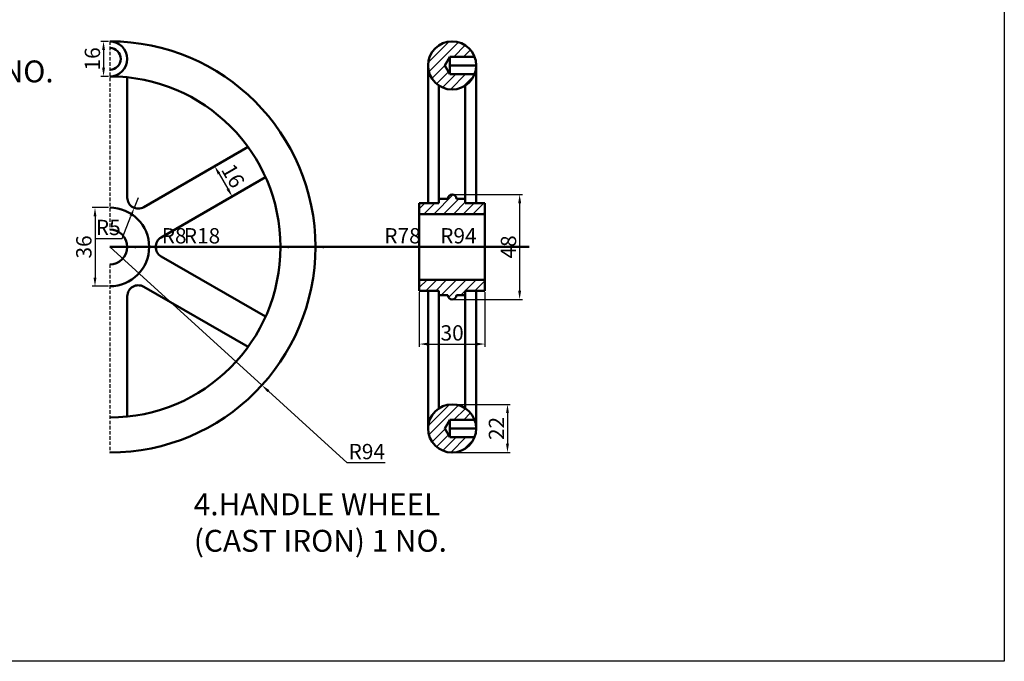
# Model space of a CAD drawing. Units: millimetres. Extents: x -66 to 1195, y -396 to 398.
# Tile 6 of 8: x 745 to 1195, y -396 to -102. Entities that reach past the tile are written whole.
import ezdxf

# ---------------------------------------------------------------- set-up
doc = ezdxf.new("R2010")
doc.units = ezdxf.units.MM
doc.header["$LTSCALE"] = 0.5
doc.linetypes.add('HIDDEN', pattern=[9.525, 6.35, -3.175])
for name, color, linetype, lineweight in [('M-DIMS', 2, 'Continuous', 25), ('M-HATC', 8, 'Continuous', 18), ('M-HIDN', 3, 'HIDDEN', 25), ('M-OUTL', 7, 'Continuous', 50), ('M-TEXT', 7, 'Continuous', 25), ('M-TTLB', 7, 'Continuous', 25)]:
    doc.layers.add(name, color=color, linetype=linetype, lineweight=lineweight)
doc.styles.get("Standard").update_dxf_attribs({"font": 'arial.ttf'})
doc.dimstyles.new('ISO-25', dxfattribs={"dimtxt": 7, "dimasz": 4, "dimexe": 1.25, "dimexo": 0.625, "dimtad": 1, "dimtoh": 1, "dimtxsty": 'Standard', "dimcen": 2.5, "dimadec": 0, "dimazin": 0, "dimtfac": 1, "dimtmove": 0, "dimatfit": 3, "dimfxl": 1, "dimarcsym": 0})

# ---------------------------------------------------------------- blocks, each defined once
blk = doc.blocks.new('*D89')
at = {"layer": 'Defpoints', "color": 0, "ltscale": 0.5, "transparency": 16777216}
for p in [(942.6, -182.22), (942.6, -230.22), (973.48, -230.22)]:
    blk.add_point(p, dxfattribs=at)
at = {"layer": 'M-DIMS', "color": 0, "lineweight": -2, "ltscale": 0.5, "transparency": 16777216}
for p, q in [((943.23, -182.22), (974.73, -182.22)), ((973.48, -186.22), (973.48, -226.22)), ((943.23, -230.22), (974.73, -230.22))]:
    blk.add_line(p, q, dxfattribs=at)
at = {"layer": 'M-DIMS', "color": 0, "ltscale": 0.5, "transparency": 16777216}
for points in [[(972.81, -186.22), (974.15, -186.22), (973.48, -182.22)], [(972.81, -226.22), (974.15, -226.22), (973.48, -230.22)]]:
    blk.add_solid(points, dxfattribs=at)
at = {"layer": 'M-DIMS', "color": 0, "ltscale": 0.5, "transparency": 16777216, "insert": (969.28, -206.22), "char_height": 7, "attachment_point": 5, "rotation": 90}
blk.add_mtext('48', dxfattribs=at)
blk = doc.blocks.new('*D90')
at = {"layer": 'Defpoints', "color": 0, "ltscale": 0.5, "transparency": 16777216}
for p in [(927.6, -226.22), (957.6, -226.22), (957.6, -250.62)]:
    blk.add_point(p, dxfattribs=at)
at = {"layer": 'M-DIMS', "color": 0, "lineweight": -2, "ltscale": 0.5, "transparency": 16777216}
for p, q in [((927.6, -226.84), (927.6, -251.87)), ((957.6, -226.84), (957.6, -251.87)), ((931.6, -250.62), (953.6, -250.62))]:
    blk.add_line(p, q, dxfattribs=at)
at = {"layer": 'M-DIMS', "color": 0, "ltscale": 0.5, "transparency": 16777216}
for points in [[(931.6, -249.95), (931.6, -251.28), (927.6, -250.62)], [(953.6, -249.95), (953.6, -251.28), (957.6, -250.62)]]:
    blk.add_solid(points, dxfattribs=at)
at = {"layer": 'M-DIMS', "color": 0, "ltscale": 0.5, "transparency": 16777216, "insert": (942.6, -246.42), "char_height": 7, "attachment_point": 5}
blk.add_mtext('30', dxfattribs=at)
blk = doc.blocks.new('*D91')
at = {"layer": 'Defpoints', "color": 0, "ltscale": 0.5, "transparency": 16777216}
for p in [(942.6, -278.22), (942.6, -300.22), (967.92, -300.22)]:
    blk.add_point(p, dxfattribs=at)
at = {"layer": 'M-DIMS', "color": 0, "lineweight": -2, "ltscale": 0.5, "transparency": 16777216}
for p, q in [((943.23, -278.22), (969.17, -278.22)), ((967.92, -282.22), (967.92, -296.22)), ((943.23, -300.22), (969.17, -300.22))]:
    blk.add_line(p, q, dxfattribs=at)
at = {"layer": 'M-DIMS', "color": 0, "ltscale": 0.5, "transparency": 16777216}
for points in [[(967.25, -282.22), (968.58, -282.22), (967.92, -278.22)], [(967.25, -296.22), (968.58, -296.22), (967.92, -300.22)]]:
    blk.add_solid(points, dxfattribs=at)
at = {"layer": 'M-DIMS', "color": 0, "ltscale": 0.5, "transparency": 16777216, "insert": (963.78, -289.22), "char_height": 7, "attachment_point": 5, "rotation": 90}
blk.add_mtext('22', dxfattribs=at)
blk = doc.blocks.new('*D92')
at = {"layer": 'Defpoints', "color": 0, "ltscale": 0.5, "transparency": 16777216}
for p in [(786.1, -206.22), (855.65, -269.46)]:
    blk.add_point(p, dxfattribs=at)
at = {"layer": 'M-DIMS', "color": 0, "lineweight": -2, "ltscale": 0.5, "transparency": 16777216}
for p, q in [((786.1, -206.22), (855.65, -269.46)), ((894.62, -304.9), (858.61, -272.15)), ((911.94, -304.9), (894.62, -304.9))]:
    blk.add_line(p, q, dxfattribs=at)
at = {"layer": 'M-DIMS', "color": 0, "ltscale": 0.5, "transparency": 16777216}
blk.add_solid([(859.05, -271.66), (858.16, -272.64), (855.65, -269.46)], dxfattribs=at)
at = {"layer": 'M-DIMS', "color": 0, "ltscale": 0.5, "transparency": 16777216, "insert": (903.59, -300.7), "char_height": 7, "attachment_point": 5}
blk.add_mtext('R94', dxfattribs=at)
blk = doc.blocks.new('*D93')
at = {"layer": 'Defpoints', "color": 0, "ltscale": 0.5, "transparency": 16777216}
for p in [(825.45, -174.26), (842.05, -183.15), (833.45, -188.12)]:
    blk.add_point(p, dxfattribs=at)
at = {"layer": 'M-DIMS', "color": 0, "lineweight": -2, "ltscale": 0.5, "transparency": 16777216}
for p, q in [((825.99, -173.95), (835.13, -168.67)), ((836.05, -172.76), (840.05, -179.69)), ((833.99, -187.81), (843.13, -182.53))]:
    blk.add_line(p, q, dxfattribs=at)
at = {"layer": 'M-DIMS', "color": 0, "ltscale": 0.5, "transparency": 16777216}
for points in [[(836.63, -172.43), (835.47, -173.1), (834.05, -169.3)], [(840.63, -179.36), (839.47, -180.02), (842.05, -183.15)]]:
    blk.add_solid(points, dxfattribs=at)
at = {"layer": 'M-DIMS', "color": 0, "ltscale": 0.5, "transparency": 16777216, "insert": (841.69, -174.13), "char_height": 7, "attachment_point": 5, "rotation": 300}
blk.add_mtext('16', dxfattribs=at)
blk = doc.blocks.new('*D94')
at = {"layer": 'Defpoints', "color": 0, "ltscale": 0.5, "transparency": 16777216}
for p in [(786.1, -188.22), (779.34, -224.22), (786.1, -224.22)]:
    blk.add_point(p, dxfattribs=at)
at = {"layer": 'M-DIMS', "color": 0, "lineweight": -2, "ltscale": 0.5, "transparency": 16777216}
for p, q in [((785.48, -188.22), (778.09, -188.22)), ((779.34, -192.22), (779.34, -220.22)), ((785.48, -224.22), (778.09, -224.22))]:
    blk.add_line(p, q, dxfattribs=at)
at = {"layer": 'M-DIMS', "color": 0, "ltscale": 0.5, "transparency": 16777216}
for points in [[(778.67, -192.22), (780, -192.22), (779.34, -188.22)], [(778.67, -220.22), (780, -220.22), (779.34, -224.22)]]:
    blk.add_solid(points, dxfattribs=at)
at = {"layer": 'M-DIMS', "color": 0, "ltscale": 0.5, "transparency": 16777216, "insert": (775.14, -206.22), "char_height": 7, "attachment_point": 5, "rotation": 90}
blk.add_mtext('36', dxfattribs=at)
blk = doc.blocks.new('*D95')
at = {"layer": 'Defpoints', "color": 0, "ltscale": 0.5, "transparency": 16777216}
for p in [(786.1, -112.22), (783.24, -128.22), (786.1, -128.22)]:
    blk.add_point(p, dxfattribs=at)
at = {"layer": 'M-DIMS', "color": 0, "lineweight": -2, "ltscale": 0.5, "transparency": 16777216}
for p, q in [((785.48, -112.22), (781.99, -112.22)), ((783.24, -116.22), (783.24, -124.22)), ((785.48, -128.22), (781.99, -128.22))]:
    blk.add_line(p, q, dxfattribs=at)
at = {"layer": 'M-DIMS', "color": 0, "ltscale": 0.5, "transparency": 16777216}
for points in [[(782.58, -116.22), (783.91, -116.22), (783.24, -112.22)], [(782.58, -124.22), (783.91, -124.22), (783.24, -128.22)]]:
    blk.add_solid(points, dxfattribs=at)
at = {"layer": 'M-DIMS', "color": 0, "ltscale": 0.5, "transparency": 16777216, "insert": (779.05, -120.22), "char_height": 7, "attachment_point": 5, "rotation": 90}
blk.add_mtext('16', dxfattribs=at)
blk = doc.blocks.new('*D125')
at = {"layer": 'Defpoints', "color": 0, "ltscale": 0.5, "transparency": 16777216}
for p in [(786.1, -206.22), (880.1, -206.22)]:
    blk.add_point(p, dxfattribs=at)
at = {"layer": 'M-DIMS', "color": 0, "lineweight": -2, "ltscale": 0.5, "transparency": 16777216}
for p, q in [((786.1, -206.22), (880.1, -206.22)), ((936.5, -206.22), (884.1, -206.22)), ((953.82, -206.22), (936.5, -206.22))]:
    blk.add_line(p, q, dxfattribs=at)
at = {"layer": 'M-DIMS', "color": 0, "ltscale": 0.5, "transparency": 16777216}
blk.add_solid([(884.1, -205.55), (884.1, -206.89), (880.1, -206.22)], dxfattribs=at)
at = {"layer": 'M-DIMS', "color": 0, "ltscale": 0.5, "transparency": 16777216, "insert": (945.47, -202.02), "char_height": 7, "attachment_point": 5}
blk.add_mtext('R94', dxfattribs=at)
blk = doc.blocks.new('*D126')
at = {"layer": 'Defpoints', "color": 0, "ltscale": 0.5, "transparency": 16777216}
for p in [(786.1, -206.22), (864.1, -206.22)]:
    blk.add_point(p, dxfattribs=at)
at = {"layer": 'M-DIMS', "color": 0, "lineweight": -2, "ltscale": 0.5, "transparency": 16777216}
for p, q in [((786.1, -206.22), (864.1, -206.22)), ((910.9, -206.22), (868.1, -206.22)), ((928.27, -206.22), (910.9, -206.22))]:
    blk.add_line(p, q, dxfattribs=at)
at = {"layer": 'M-DIMS', "color": 0, "ltscale": 0.5, "transparency": 16777216}
blk.add_solid([(868.1, -205.55), (868.1, -206.89), (864.1, -206.22)], dxfattribs=at)
at = {"layer": 'M-DIMS', "color": 0, "ltscale": 0.5, "transparency": 16777216, "insert": (919.9, -202.02), "char_height": 7, "attachment_point": 5}
blk.add_mtext('R78', dxfattribs=at)
blk = doc.blocks.new('*D127')
at = {"layer": 'Defpoints', "color": 0, "ltscale": 0.5, "transparency": 16777216}
for p in [(786.1, -206.22), (804.1, -206.22)]:
    blk.add_point(p, dxfattribs=at)
at = {"layer": 'M-DIMS', "color": 0, "lineweight": -2, "ltscale": 0.5, "transparency": 16777216}
for p, q in [((786.1, -206.22), (804.1, -206.22)), ((819.25, -206.22), (808.1, -206.22)), ((836.61, -206.22), (819.25, -206.22))]:
    blk.add_line(p, q, dxfattribs=at)
at = {"layer": 'M-DIMS', "color": 0, "ltscale": 0.5, "transparency": 16777216}
blk.add_solid([(808.1, -205.55), (808.1, -206.89), (804.1, -206.22)], dxfattribs=at)
at = {"layer": 'M-DIMS', "color": 0, "ltscale": 0.5, "transparency": 16777216, "insert": (828.24, -202.02), "char_height": 7, "attachment_point": 5}
blk.add_mtext('R18', dxfattribs=at)
blk = doc.blocks.new('*D128')
at = {"layer": 'Defpoints', "color": 0, "ltscale": 0.5, "transparency": 16777216}
for p in [(786.1, -206.22), (794.1, -206.22)]:
    blk.add_point(p, dxfattribs=at)
at = {"layer": 'M-DIMS', "color": 0, "lineweight": -2, "ltscale": 0.5, "transparency": 16777216}
for p, q in [((786.1, -206.22), (794.1, -206.22)), ((809.25, -206.22), (798.1, -206.22)), ((821.18, -206.22), (809.25, -206.22))]:
    blk.add_line(p, q, dxfattribs=at)
at = {"layer": 'M-DIMS', "color": 0, "ltscale": 0.5, "transparency": 16777216}
blk.add_solid([(798.1, -205.55), (798.1, -206.89), (794.1, -206.22)], dxfattribs=at)
at = {"layer": 'M-DIMS', "color": 0, "ltscale": 0.5, "transparency": 16777216, "insert": (815.53, -202.02), "char_height": 7, "attachment_point": 5}
blk.add_mtext('R8', dxfattribs=at)
blk = doc.blocks.new('*D129')
at = {"layer": 'Defpoints', "color": 0, "ltscale": 0.5, "transparency": 16777216}
for p in [(799.1, -183.7), (797.26, -188.35)]:
    blk.add_point(p, dxfattribs=at)
at = {"layer": 'M-DIMS', "color": 0, "lineweight": -2, "ltscale": 0.5, "transparency": 16777216}
for p, q in [((799.1, -183.7), (797.26, -188.35)), ((791.68, -202.4), (795.78, -192.07)), ((779.72, -202.4), (791.68, -202.4))]:
    blk.add_line(p, q, dxfattribs=at)
at = {"layer": 'M-DIMS', "color": 0, "ltscale": 0.5, "transparency": 16777216}
blk.add_solid([(795.16, -191.82), (796.4, -192.31), (797.26, -188.35)], dxfattribs=at)
at = {"layer": 'M-DIMS', "color": 0, "ltscale": 0.5, "transparency": 16777216, "insert": (785.39, -198.22), "char_height": 7, "attachment_point": 5}
blk.add_mtext('R5', dxfattribs=at)

msp = doc.modelspace()

# ---------------------------------------------------------------- hatches: boundary and pattern name
at = {"layer": 'M-HATC', "ltscale": 0.5}
h = msp.add_hatch(dxfattribs=at)
h.set_pattern_fill('ANSI31', color=256)
h.set_pattern_definition([(45, (-907.1492, -38.9293), (-2.245064, 2.245064), [])])
h.paths.add_polyline_path([(957.6042, -191.2187), (957.6042, -186.2187), (948.6042, -186.2187), (948.6042, -184.2187), (944.6042, -184.2187, 1), (940.6042, -184.2187), (936.6042, -184.2187), (936.6042, -186.2187), (927.6042, -186.2187), (927.6042, -191.2187)])
h.paths.add_polyline_path([(948.6042, -228.2187), (948.6042, -226.2187), (957.6042, -226.2187), (957.6042, -221.2187), (927.6042, -221.2187), (927.6042, -226.2187), (936.6042, -226.2187), (936.6042, -228.2187), (940.6042, -228.2187, 1), (944.6042, -228.2187)])
h.paths.add_polyline_path([(931.6042, -123.2187, 0.41421356), (942.6042, -134.2187, 0.30896041), (952.8511, -127.2187), (941.6042, -127.2187), (939.2948, -123.2187), (941.6042, -119.2187), (952.8511, -119.2187, 0.82930474)])
h.paths.add_polyline_path([(941.6042, -285.2187), (952.8511, -285.2187, 0.30896041), (942.6042, -278.2187, 0.41421356), (931.6042, -289.2187, 0.82930474), (952.8511, -293.2187), (941.6042, -293.2187), (939.2948, -289.2187)])

# ---------------------------------------------------------------- linework, layer by layer
at = {"layer": 'M-HIDN', "ltscale": 0.5}
for p, q in [((786.101, -112.2187), (786.101, -198.2187)), ((786.101, -214.2187), (786.101, -300.2187))]:
    msp.add_line(p, q, dxfattribs=at)
at = {"layer": 'M-OUTL', "ltscale": 0.5}
for p, q in [((941.6042, -119.2187), (939.2948, -123.2187)), ((941.6042, -123.2187), (941.6042, -119.2187)), ((941.6042, -119.2187), (952.8511, -119.2187)), ((931.6042, -123.2187), (931.6042, -186.2187)), ((941.6042, -127.2187), (939.2948, -123.2187)), ((953.6042, -123.2187), (941.6042, -123.2187)), ((941.6042, -123.2187), (941.6042, -127.2187)), ((953.6042, -123.2187), (953.6042, -186.2187)), ((794.101, -183.7021), (794.101, -128.6301)), ((941.6042, -127.2187), (953.6042, -127.2187)), ((936.6042, -184.2187), (936.6042, -132.4383)), ((948.6042, -184.2187), (948.6042, -132.4383)), ((801.601, -188.0322), (849.2947, -160.4962)), ((809.601, -201.8886), (857.2947, -174.3526)), ((936.6042, -184.2187), (936.6042, -186.2187)), ((936.6042, -184.2187), (940.6042, -184.2187)), ((944.6042, -184.2187), (948.6042, -184.2187)), ((948.6042, -184.2187), (948.6042, -186.2187)), ((927.6042, -186.2187), (927.6042, -206.2187)), ((936.6042, -186.2187), (927.6042, -186.2187)), ((957.6042, -186.2187), (948.6042, -186.2187)), ((957.6042, -206.2187), (957.6042, -186.2187)), ((957.6042, -191.2187), (927.6042, -191.2187)), ((786.101, -206.2187), (977.7534, -206.2187)), ((927.6042, -226.2187), (927.6042, -206.2187)), ((957.6042, -206.2187), (957.6042, -226.2187)), ((809.601, -210.5488), (857.2947, -238.0848)), ((801.601, -224.4052), (849.2947, -251.9412)), ((957.6042, -221.2187), (927.6042, -221.2187)), ((794.101, -228.7354), (794.101, -283.8074)), ((936.6042, -226.2187), (927.6042, -226.2187)), ((931.6042, -289.2187), (931.6042, -226.2187)), ((936.6042, -228.2187), (936.6042, -226.2187)), ((936.6042, -228.2187), (936.6042, -279.9992)), ((936.6042, -228.2187), (940.6042, -228.2187)), ((944.6042, -228.2187), (948.6042, -228.2187)), ((957.6042, -226.2187), (948.6042, -226.2187)), ((948.6042, -228.2187), (948.6042, -226.2187)), ((948.6042, -228.2187), (948.6042, -279.9992)), ((953.6042, -289.2187), (953.6042, -226.2187)), ((941.6042, -285.2187), (939.2948, -289.2187)), ((941.6042, -289.2187), (941.6042, -285.2187)), ((941.6042, -285.2187), (953.6042, -285.2187)), ((941.6042, -293.2187), (939.2948, -289.2187)), ((953.6042, -289.2187), (941.6042, -289.2187)), ((941.6042, -289.2187), (941.6042, -293.2187)), ((941.6042, -293.2187), (952.8511, -293.2187))]:
    msp.add_line(p, q, dxfattribs=at)
for centre, radius, start, end in [((786.101, -206.2187), 94, 270, 90), ((786.101, -120.2187), 8, 270, 90), ((942.6042, -123.2187), 11, 270, 180), ((786.101, -120.2187), 5, 270, 90), ((942.6042, -123.2187), 11, 180, 270), ((786.101, -206.2187), 78, 270, 90), ((799.101, -183.7021), 5, 180, 300), ((942.6042, -184.2187), 2, 0, 180), ((786.101, -206.2187), 18, 270, 90), ((786.101, -206.2187), 8, 270, 90), ((812.101, -206.2187), 5, 120, 240), ((799.101, -228.7354), 5, 60, 180), ((942.6042, -228.2187), 2, 180, 0), ((942.6042, -289.2187), 11, 180, 90), ((942.6042, -289.2187), 11, 90, 180)]:
    msp.add_arc(centre, radius, start, end, dxfattribs=at)
at = {"layer": 'M-TTLB', "ltscale": 0.5}
msp.add_lwpolyline([(-66.4176, 397.641), (1195.0519, 397.641), (1195.0519, -395.6964), (-66.4176, -395.6964)], close=True, dxfattribs=at)

# ---------------------------------------------------------------- texts
at = {"layer": 'M-TEXT', "ltscale": 0.5, "char_height": 10, "attachment_point": 1}
for s, width, insert in [('\\pxqc;10.KEY\\P (MILD STEEL) 1 NO.', 203.992441, (596.2267, -104.2757)), ('\\pxqc;4.HANDLE WHEEL\\P (CAST IRON) 1 NO.', 191.333714, (785.1682, -318.9122))]:
    msp.add_mtext_dynamic_manual_height_columns(s, width=width, gutter_width=12.5, heights=[0], dxfattribs=dict(at, insert=insert))

# ---------------------------------------------------------------- dimensions: what is measured, and where the dimension line sits
at = {"layer": 'M-DIMS', "ltscale": 0.5}
for base, p1, p2, picture, middle in [((783.2447, -128.2187), (786.101, -112.2187), (786.101, -128.2187), '*D95', (779.0457, -120.2187)), ((973.4813, -230.2187), (942.6042, -182.2187), (942.6042, -230.2187), '*D89', (969.2823, -206.2187)), ((779.3369, -224.2187), (786.101, -188.2187), (786.101, -224.2187), '*D94', (775.1355, -206.2187)), ((967.918, -300.2187), (942.6042, -278.2187), (942.6042, -300.2187), '*D91', (963.7787, -289.2187))]:
    dim = msp.add_linear_dim(base=base, p1=p1, p2=p2, angle=90, dimstyle='ISO-25', override={"dimclrd": 0, "dimclre": 0, "dimclrt": 0}, dxfattribs=at)
    dim.commit()
    dim.dimension.update_dxf_attribs({"geometry": picture, "text_midpoint": middle})
dim = msp.add_aligned_dim(p1=(825.4479, -174.2642), p2=(833.4479, -188.1206), distance=9.9325, dimstyle='ISO-25', override={"dimclrd": 0, "dimclre": 0, "dimclrt": 0}, dxfattribs=at)
dim.commit()
dim.dimension.update_dxf_attribs({"geometry": '*D93', "text_midpoint": (841.6861, -174.1266)})
for center, mpoint, picture, middle in [((799.101, -183.7021), (797.2578, -188.3499), '*D129', (785.389, -198.2198)), ((786.101, -206.2187), (804.101, -206.22), '*D127', (828.2444, -202.0221)), ((786.101, -206.2187), (794.101, -206.22), '*D128', (815.5251, -202.0234))]:
    dim = msp.add_radius_dim(center=center, mpoint=mpoint, dimstyle='ISO-25', override={"dimdec": 0, "dimlfac": 1, "dimrnd": 0, "dimzin": 0, "dimdsep": 46, "dimlunit": 2}, dxfattribs=at)
    dim.commit()
    dim.dimension.update_dxf_attribs({"geometry": picture, "text_midpoint": middle})
for mpoint, override, picture, middle in [((880.101, -206.22), {"dimdec": 0, "dimlfac": 1, "dimrnd": 0, "dimzin": 0, "dimdsep": 46, "dimlunit": 2}, '*D125', (936.501, -206.2208)), ((864.101, -206.22), {"dimdec": 0, "dimlfac": 1, "dimrnd": 0, "dimzin": 0, "dimdsep": 46, "dimlunit": 2}, '*D126', (910.901, -206.2208)), ((855.6467, -269.4595), {"dimclrd": 0, "dimclre": 0, "dimclrt": 0}, '*D92', (903.5947, -304.9003))]:
    dim = msp.add_radius_dim(center=(786.101, -206.2187), mpoint=mpoint, dimstyle='ISO-25', override=override, dxfattribs=at)
    dim.commit()
    dim.dimension.update_dxf_attribs({"geometry": picture, "text_midpoint": middle, "dimtype": 164})
dim = msp.add_linear_dim(base=(957.6042, -250.618), p1=(927.6042, -226.2187), p2=(957.6042, -226.2187), dimstyle='ISO-25', override={"dimclrd": 0, "dimclre": 0, "dimclrt": 0}, dxfattribs=at)
dim.commit()
dim.dimension.update_dxf_attribs({"geometry": '*D90', "text_midpoint": (942.6042, -246.4166)})

doc.saveas('drawing.dxf')
